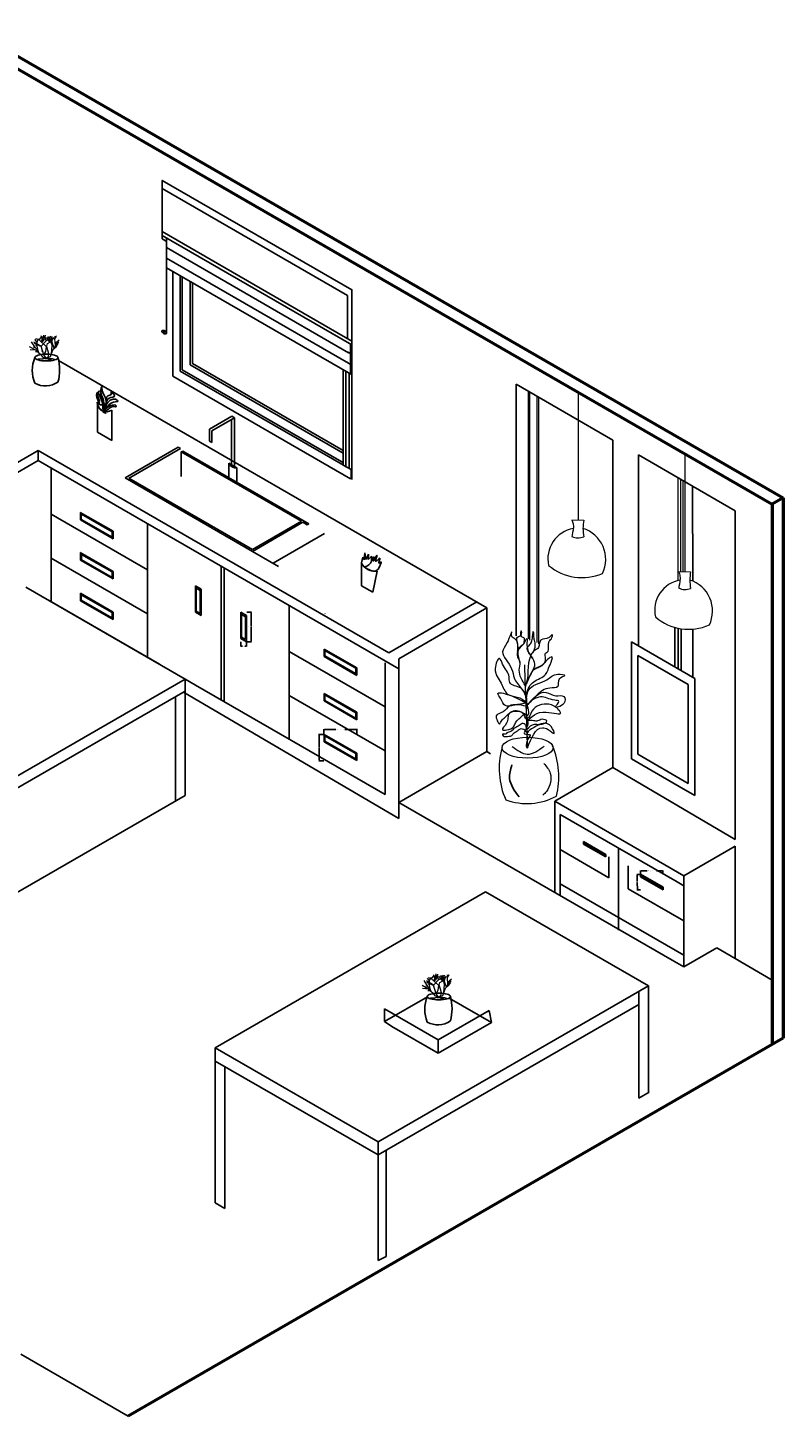
# Model space of a CAD drawing. Units: centimetres. Extents: x 5383 to 11288, y 5305 to 11515.
# Tile 4 of 5: x 5675 to 5972, y 5305 to 5851. Entities that reach past the tile are written whole.
import ezdxf

# ---------------------------------------------------------------- set-up
doc = ezdxf.new("R2010")
doc.units = ezdxf.units.CM
for name, color, linetype, lineweight in [('A-ANNO-DIMS', 2, 'Continuous', 18), ('A-FLOR-CASE', 3, 'Continuous', 25), ('A-FLOR-FIXT', 6, 'Continuous', 25), ('A-FURN', 8, 'Continuous', 25), ('A-FURN-PLNT', 82, 'Continuous', 13), ('A-GLAZ', 4, 'Continuous', 25), ('A-WALL', 7, 'Continuous', 50), ('E-LITE', 2, 'Continuous', 18)]:
    doc.layers.add(name, color=color, linetype=linetype, lineweight=lineweight)
doc.styles.get("Standard").update_dxf_attribs({"font": 'arial.ttf'})
doc.dimstyles.get("Standard").update_dxf_attribs({"dimtxt": 0.18, "dimasz": 0.18, "dimexe": 0.18, "dimexo": 0.0625, "dimgap": 0.09, "dimtad": 0, "dimtih": 1, "dimtoh": 1, "dimdec": 4, "dimzin": 0, "dimdsep": 46, "dimtxsty": 'Standard', "dimcen": 0.09, "dimadec": 0, "dimazin": 0, "dimtfac": 1, "dimtdec": 4, "dimtofl": 0, "dimtmove": 0, "dimatfit": 3, "dimfxl": 1, "dimtolj": 1, "dimtzin": 0, "dimarcsym": 0})

# ---------------------------------------------------------------- blocks, each defined once
blk = doc.blocks.new('*U2')
for p, q in [((-18.24, 11.04), (-21.755, 16.655)), ((-12.96, 12.48), (-19.68, 16.32)), ((-13.92, 12.48), (-19.2, 14.88)), ((-16.8, 16.32), (-18.72, 18.72)), ((-14.88, 18.24), (-17.76, 19.2)), ((-16.8, 12.48), (-17.76, 12.96)), ((-16.8, 16.32), (-15.36, 19.68)), ((-16.8, 12.48), (-16.8, 16.32)), ((-14.88, 18.24), (-12.96, 20.64)), ((-8.16, 12), (-14.88, 18.24)), ((-13.325, 16.724), (-11.433, 18.289)), ((-12.96, 12.48), (-8.16, 17.76)), ((-12.471, 19.775), (-12.898, 22.044)), ((-11.677, 19.071), (-12.471, 19.775)), ((-11.28, 19.619), (-12.104, 21.184)), ((-12.043, 15.628), (-11.921, 18.836)), ((-11.982, 16.802), (-10.579, 18.054)), ((-11.921, 18.836), (-10.64, 20.401)), ((-11.433, 18.289), (-10.457, 22.749)), ((-10.579, 18.054), (-9.846, 19.697)), ((-8.16, 17.76), (-10.56, 21.6)), ((-9.48, 19.775), (-8.992, 22.592)), ((-7.2, 19.68), (-8.64, 20.16)), ((-8.16, 17.76), (-5.28, 19.2)), ((-7.68, 12.48), (-7.2, 14.88)), ((-7.2, 19.68), (-6.24, 21.12)), ((-4.8, 16.32), (-7.2, 19.68)), ((-7.2, 14.88), (-3.84, 16.8)), ((-5.086, 17.741), (-5.513, 21.34)), ((-5.28, 19.2), (-3.84, 21.6)), ((-3.377, 15.315), (-5.086, 17.819)), ((-2.88, 12.96), (-4.32, 19.68)), ((-3.84, 16.8), (-0.96, 20.64)), ((-3.377, 18.602), (-2.888, 21.575)), ((-2.766, 16.802), (-3.377, 18.602)), ((-3.36, 5.28), (-2.88, 12.96)), ((-2.88, 15.84), (-2.4, 20.16)), ((-0.96, 10.56), (-2.88, 15.84)), ((-0.508, 21.888), (-0.081, 20.558)), ((-0.48, 10.8), (0.346, 13.203)), ((-0.203, 19.149), (0.102, 21.34)), ((0.346, 13.203), (-0.203, 19.149)), ((-0.142, 19.384), (0.59, 20.401)), ((-0.02, 20.01), (0.896, 21.105)), ((0.041, 20.714), (1.384, 22.044)), ((0.102, 21.34), (0.835, 21.888)), ((0.346, 13.203), (1.323, 16.254)), ((0.96, 12), (1.44, 15.36)), ((0.96, 12), (2.88, 14.88)), ((1.323, 16.254), (3.642, 18.289)), ((1.44, 15.36), (2.88, 17.28)), ((1.92, 13.44), (2.4, 15.36)), ((2.4, 15.36), (3.36, 16.32)), ((-17.76, 8.64), (-23.663, 11.961)), ((-17.76, 8.64), (-23.128, 9.222)), ((-18.24, 11.04), (-20.16, 11.52)), ((-15.84, 8.16), (-18.24, 11.04)), ((-16.32, 7.2), (-18.24, 7.2)), ((-14.88, 5.76), (-17.76, 8.64)), ((-15.84, 0.48), (-17.76, 0)), ((-15.84, 8.16), (-16.8, 12.48)), ((-14.88, 5.76), (-15.84, 8.16)), ((-13.44, 0.48), (-15.84, 0.48)), ((-12.96, 4.8), (-14.88, 5.76)), ((-12.96, 12.48), (-13.92, 12.48)), ((-9.6, 0.96), (-13.44, 0.48)), ((-10.56, 4.32), (-12.96, 12.48)), ((-11.52, 2.4), (-12.96, 4.8)), ((-9.6, 0.96), (-12.96, 0)), ((-8.64, 0.96), (-11.52, 2.4)), ((-10.56, 4.32), (-8.64, 7.68)), ((-8.64, 1.92), (-10.56, 4.32)), ((-9.6, 0.96), (-7.68, 0.96)), ((-8.64, 7.68), (-8.16, 12)), ((-8.64, 0.96), (-4.32, 2.88)), ((-8.64, 0.96), (-6.24, 2.88)), ((-8.64, 0.96), (-8.64, 1.92)), ((-8.64, 0.96), (-2.88, 0.96)), ((-6.72, 8.64), (-7.68, 12.48)), ((-7.68, 0.96), (-6.24, 0.48)), ((-5.76, 5.28), (-6.72, 8.64)), ((-6.24, 2.88), (-5.76, 5.28)), ((-6.24, 0.48), (-3.36, 0)), ((-4.32, 2.88), (-1.92, 9.6)), ((-2.88, 0.96), (0, 0)), ((-1.92, 9.6), (0.96, 12))]:
    blk.add_line(p, q)
blk = doc.blocks.new('HANDLE-DRAWER')
for p, q in [((12.85, 2.94), (0, 10.36)), ((0.01, 7.41), (0.01, 10.35)), ((0.01, 7.41), (12.85, 0)), ((0.4, 7.58), (0.4, 9.71)), ((12.49, 0.59), (0.4, 7.58)), ((0.5, 9.66), (12.49, 2.73)), ((12.49, 2.73), (12.49, 0.59)), ((12.85, 0), (12.85, 2.94))]:
    blk.add_line(p, q)
blk = doc.blocks.new('HANDLE-DRAWER-B')
for p, q in [((0, 6.1), (8.78, 1.03)), ((0, 6.1), (0, 5.07)), ((0.19, 5.78), (8.61, 0.92)), ((0.19, 5.78), (0.19, 5.23)), ((8.78, 0), (0, 5.07)), ((8.61, 0.37), (0.19, 5.23)), ((8.61, 0.92), (8.61, 0.37)), ((8.78, 1.03), (8.78, 0))]:
    blk.add_line(p, q)
blk = doc.blocks.new('HANDLE-DOOR-D')
for p, q in [((0, 11.69), (2.28, 10.37)), ((0, 1.32), (0, 11.69)), ((0.33, 10.73), (1.92, 9.81)), ((0.33, 1.75), (0.33, 10.73)), ((1.92, 9.81), (1.92, 0.83)), ((2.28, 10.37), (2.28, 0)), ((2.28, 0), (0, 1.32)), ((1.92, 0.83), (0.33, 1.75))]:
    blk.add_line(p, q)
blk = doc.blocks.new('*D16')
at = {"layer": 'A-ANNO-DIMS', "color": 0, "lineweight": -2, "transparency": 16777216}
for p, q in [((5791.14, 5573.38), (5791.14, 5575.42)), ((5791.32, 5575.24), (5795.82, 5575.25)), ((5803.82, 5575.25), (5799.32, 5575.25)), ((5804, 5573.39), (5804, 5575.43))]:
    blk.add_line(p, q, dxfattribs=at)
at = {"layer": 'A-ANNO-DIMS', "color": 0, "transparency": 16777216}
for points in [[(5791.32, 5575.27), (5791.32, 5575.21), (5791.14, 5575.24)], [(5803.82, 5575.28), (5803.82, 5575.22), (5804, 5575.25)]]:
    blk.add_solid(points, dxfattribs=at)
at = {"layer": 'Defpoints', "color": 0, "transparency": 16777216}
for p in [(5791.14, 5575.24), (5791.14, 5573.32), (5804, 5573.33)]:
    blk.add_point(p, dxfattribs=at)
at = {"layer": 'A-ANNO-DIMS', "color": 0, "transparency": 16777216, "insert": (5797.57, 5575.25), "char_height": 0.18, "attachment_point": 5}
blk.add_mtext('\\A1;HANDLE (DRAWER) 13 TYP.', dxfattribs=at)
blk = doc.blocks.new('*D17')
at = {"layer": 'A-ANNO-DIMS', "color": 0, "lineweight": -2, "transparency": 16777216}
for p, q in [((5791.08, 5573.32), (5789.04, 5573.31)), ((5789.22, 5573.13), (5789.22, 5568.32)), ((5789.22, 5563.13), (5789.22, 5567.95)), ((5791.09, 5562.96), (5789.05, 5562.95))]:
    blk.add_line(p, q, dxfattribs=at)
at = {"layer": 'A-ANNO-DIMS', "color": 0, "transparency": 16777216}
for points in [[(5789.25, 5573.13), (5789.19, 5573.13), (5789.22, 5573.31)], [(5789.25, 5563.13), (5789.19, 5563.13), (5789.23, 5562.95)]]:
    blk.add_solid(points, dxfattribs=at)
at = {"layer": 'Defpoints', "color": 0, "transparency": 16777216}
for p in [(5791.14, 5573.32), (5789.23, 5562.95), (5791.15, 5562.96)]:
    blk.add_point(p, dxfattribs=at)
at = {"layer": 'A-ANNO-DIMS', "color": 0, "transparency": 16777216, "insert": (5789.22, 5568.13), "char_height": 0.18, "attachment_point": 5}
blk.add_mtext('\\A1;10 TYP.', dxfattribs=at)
blk = doc.blocks.new('*D24')
at = {"layer": 'A-ANNO-DIMS', "color": 0, "lineweight": -2, "transparency": 16777216}
for p, q in [((5915.66, 5518.31), (5915.66, 5519.74)), ((5915.84, 5519.56), (5918.25, 5519.57)), ((5924.26, 5519.61), (5921.84, 5519.59)), ((5924.44, 5518.35), (5924.44, 5519.79))]:
    blk.add_line(p, q, dxfattribs=at)
at = {"layer": 'A-ANNO-DIMS', "color": 0, "transparency": 16777216}
for points in [[(5915.84, 5519.59), (5915.84, 5519.53), (5915.66, 5519.56)], [(5924.26, 5519.64), (5924.26, 5519.58), (5924.44, 5519.61)]]:
    blk.add_solid(points, dxfattribs=at)
at = {"layer": 'Defpoints', "color": 0, "transparency": 16777216}
for p in [(5915.66, 5519.56), (5915.66, 5518.24), (5924.44, 5518.29)]:
    blk.add_point(p, dxfattribs=at)
at = {"layer": 'A-ANNO-DIMS', "color": 0, "transparency": 16777216, "insert": (5920.05, 5519.58), "char_height": 0.18, "attachment_point": 5}
blk.add_mtext('\\A1;HANDLE (DRAWER B) 9 TYP.', dxfattribs=at)
blk = doc.blocks.new('*D25')
at = {"layer": 'A-ANNO-DIMS', "color": 0, "lineweight": -2, "transparency": 16777216}
for p, q in [((5915.6, 5518.24), (5914.17, 5518.23)), ((5914.35, 5518.06), (5914.36, 5515.37)), ((5914.38, 5512.32), (5914.36, 5515.01)), ((5915.63, 5512.15), (5914.2, 5512.14))]:
    blk.add_line(p, q, dxfattribs=at)
at = {"layer": 'A-ANNO-DIMS', "color": 0, "transparency": 16777216}
for points in [[(5914.38, 5518.06), (5914.32, 5518.06), (5914.35, 5518.24)], [(5914.41, 5512.32), (5914.35, 5512.32), (5914.38, 5512.14)]]:
    blk.add_solid(points, dxfattribs=at)
at = {"layer": 'Defpoints', "color": 0, "transparency": 16777216}
for p in [(5915.66, 5518.24), (5914.38, 5512.14), (5915.7, 5512.15)]:
    blk.add_point(p, dxfattribs=at)
at = {"layer": 'A-ANNO-DIMS', "color": 0, "transparency": 16777216, "insert": (5914.36, 5515.19), "char_height": 0.18, "attachment_point": 5}
blk.add_mtext('\\A1;6 TYP.', dxfattribs=at)
blk = doc.blocks.new('*D26')
at = {"layer": 'A-ANNO-DIMS', "color": 0, "lineweight": -2, "transparency": 16777216}
for p, q in [((5760.76, 5621.46), (5762.63, 5621.46)), ((5762.45, 5621.28), (5762.45, 5615.79)), ((5762.45, 5609.95), (5762.45, 5615.43)), ((5760.76, 5609.77), (5762.63, 5609.77))]:
    blk.add_line(p, q, dxfattribs=at)
at = {"layer": 'A-ANNO-DIMS', "color": 0, "transparency": 16777216}
for points in [[(5762.42, 5621.28), (5762.48, 5621.28), (5762.45, 5621.46)], [(5762.42, 5609.95), (5762.48, 5609.95), (5762.45, 5609.77)]]:
    blk.add_solid(points, dxfattribs=at)
at = {"layer": 'Defpoints', "color": 0, "transparency": 16777216}
for p in [(5760.7, 5621.46), (5762.45, 5621.46), (5760.7, 5609.77)]:
    blk.add_point(p, dxfattribs=at)
at = {"layer": 'A-ANNO-DIMS', "color": 0, "transparency": 16777216, "insert": (5762.45, 5615.61), "char_height": 0.18, "attachment_point": 5}
blk.add_mtext('\\A1;HANDLE D 12 TYP.', dxfattribs=at)
blk = doc.blocks.new('*D27')
at = {"layer": 'A-ANNO-DIMS', "color": 0, "lineweight": -2, "transparency": 16777216}
for p, q in [((5758.41, 5609.71), (5758.41, 5607.84)), ((5758.59, 5608.02), (5759.09, 5608.02)), ((5760.52, 5608.02), (5760.01, 5608.02)), ((5760.7, 5609.71), (5760.7, 5607.84))]:
    blk.add_line(p, q, dxfattribs=at)
at = {"layer": 'A-ANNO-DIMS', "color": 0, "transparency": 16777216}
for points in [[(5758.59, 5608.05), (5758.59, 5607.99), (5758.41, 5608.02)], [(5760.52, 5608.05), (5760.52, 5607.99), (5760.7, 5608.02)]]:
    blk.add_solid(points, dxfattribs=at)
at = {"layer": 'Defpoints', "color": 0, "transparency": 16777216}
for p in [(5758.41, 5609.77), (5760.7, 5609.77), (5760.7, 5608.02)]:
    blk.add_point(p, dxfattribs=at)
at = {"layer": 'A-ANNO-DIMS', "color": 0, "transparency": 16777216, "insert": (5759.55, 5608.02), "char_height": 0.18, "attachment_point": 5}
blk.add_mtext('\\A1;2 TYP.', dxfattribs=at)

msp = doc.modelspace()

# ---------------------------------------------------------------- linework, layer by layer
at = {"layer": 'A-FLOR-CASE'}
for p, q in [((5678.77, 5725.01), (5678.79, 5725.03)), ((5680, 5724.33), (5680.45, 5724.06)), ((5686.8, 5720.4), (5855.22, 5623.16)), ((5866.77, 5622.62), (5866.77, 5711.16)), ((5866.77, 5711.16), (5904.77, 5689.1)), ((5702.01, 5704.03), (5702.01, 5692.28)), ((5707.72, 5688.98), (5707.72, 5700.91)), ((5702.01, 5692.28), (5707.72, 5688.98)), ((5904.77, 5686.2), (5904.77, 5689.1)), ((5575.44, 5625.3), (5678.79, 5684.97)), ((5678.79, 5681.05), (5678.79, 5684.97)), ((5678.79, 5684.97), (5816.59, 5605.41)), ((5904.77, 5686.2), (5904.77, 5560.27)), ((5914.77, 5683.3), (5914.77, 5608.1)), ((5914.77, 5683.3), (5952.78, 5661.23)), ((5575.44, 5621.38), (5678.79, 5681.05)), ((5678.79, 5681.05), (5820.61, 5599.16)), ((5683.84, 5678.13), (5683.84, 5625.49)), ((5936.1, 5670.91), (5936.17, 5633.61)), ((5683.84, 5659.91), (5721.78, 5638)), ((5708.17, 5653.2), (5695.32, 5660.62)), ((5695.33, 5657.67), (5695.33, 5660.61)), ((5695.71, 5657.83), (5695.71, 5659.97)), ((5695.71, 5659.97), (5695.81, 5659.91)), ((5695.81, 5659.91), (5707.81, 5652.99)), ((5952.78, 5661.23), (5952.78, 5531.97)), ((5695.33, 5657.67), (5708.17, 5650.26)), ((5707.81, 5650.85), (5695.71, 5657.83)), ((5721.78, 5656.22), (5721.78, 5603.58)), ((5707.81, 5652.99), (5707.81, 5650.85)), ((5708.17, 5650.26), (5708.17, 5653.2)), ((5806.95, 5641.99), (5807.23, 5644.68)), ((5807.23, 5644.68), (5807.6, 5642.18)), ((5807.6, 5642.18), (5808.68, 5644.25)), ((5808.68, 5644.25), (5808.55, 5642.08)), ((5808.55, 5642.08), (5809.86, 5643.46)), ((5809.86, 5643.46), (5809.8, 5641.5)), ((5683.84, 5642.7), (5721.78, 5620.79)), ((5750.64, 5639.56), (5750.64, 5586.92)), ((5751.89, 5638.84), (5751.89, 5586.2)), ((5805.85, 5640.82), (5806.37, 5643)), ((5805.85, 5640.82), (5805.85, 5631.8)), ((5806.37, 5643), (5806.95, 5641.99)), ((5812.07, 5637.58), (5810.32, 5629.21)), ((5673.95, 5631.2), (5736.51, 5595.08)), ((5805.85, 5631.8), (5810.32, 5629.21)), ((5683.06, 5625.94), (5726.46, 5600.88)), ((5777.44, 5624.09), (5777.44, 5571.45)), ((5816.59, 5605.41), (5851.28, 5625.44)), ((5855.22, 5623.16), (5820.61, 5603.09)), ((5855.22, 5623.16), (5855.22, 5566.51)), ((5866.77, 5622.62), (5866.77, 5612.08)), ((5791.51, 5620.82), (5791.61, 5620.76)), ((5929.1, 5615.44), (5929.1, 5599.83)), ((5930.48, 5615.1), (5930.48, 5599.03)), ((5931.63, 5614.9), (5931.63, 5598.37)), ((5936.17, 5614.74), (5936.17, 5595.75)), ((5777.44, 5605.87), (5815.15, 5584.1)), ((5936.96, 5595.29), (5912.01, 5609.7)), ((5912.01, 5609.7), (5912.01, 5563.63)), ((5815.15, 5601.43), (5815.15, 5549.68)), ((5820.61, 5603.09), (5820.61, 5599.16)), ((5914.53, 5604.41), (5934.41, 5592.93)), ((5914.53, 5565.49), (5914.53, 5604.41)), ((5736.51, 5595.08), (5620.89, 5528.33)), ((5740.66, 5592.69), (5736.22, 5595.24)), ((5736.51, 5595.08), (5738.15, 5594.13)), ((5736.51, 5595.08), (5736.51, 5549.21)), ((5820.61, 5599.16), (5820.61, 5546.52)), ((5936.96, 5549.23), (5936.96, 5595.29)), ((5620.89, 5523.54), (5736.51, 5590.29)), ((5738.15, 5588.61), (5735.87, 5589.92)), ((5740.66, 5592.69), (5815.15, 5549.68)), ((5934.41, 5592.93), (5934.41, 5554.01)), ((5732.81, 5588.15), (5732.81, 5547.08)), ((5820.61, 5540.21), (5738.15, 5588.61)), ((5777.44, 5588.66), (5815.15, 5566.89)), ((5820.61, 5546.52), (5855.22, 5566.51)), ((5855.22, 5566.51), (5856.64, 5565.68)), ((5912.01, 5563.63), (5930.86, 5552.75)), ((5934.41, 5554.01), (5914.53, 5565.49)), ((5904.77, 5560.27), (5881.87, 5547.04)), ((5904.77, 5560.27), (5952.78, 5531.97)), ((5930.86, 5552.75), (5936.96, 5549.23)), ((5640.52, 5493.8), (5736.51, 5549.21)), ((5820.61, 5546.52), (5820.61, 5540.21)), ((5820.61, 5546.52), (5928.12, 5484.45)), ((5881.87, 5547.04), (5932.67, 5517.71)), ((5881.87, 5547.04), (5881.87, 5511.16)), ((5884.02, 5541.81), (5884.02, 5509.91)), ((5884.02, 5541.81), (5929.98, 5515.28)), ((5952.78, 5529.32), (5932.67, 5517.71)), ((5952.78, 5529.32), (5952.78, 5508.19)), ((5884.02, 5528), (5903.21, 5516.93)), ((5903.21, 5516.93), (5903.21, 5525.17)), ((5907, 5528.55), (5907, 5496.32)), ((5910.7, 5512.6), (5910.7, 5521.56)), ((5884.02, 5514.52), (5932.67, 5486.43)), ((5910.7, 5512.6), (5932.67, 5499.92)), ((5929.98, 5515.28), (5932.67, 5513.73)), ((5932.67, 5517.71), (5932.67, 5481.83)), ((5952.78, 5508.19), (5952.78, 5485.1)), ((5932.67, 5481.83), (5945.56, 5489.27)), ((5952.78, 5485.1), (5945.56, 5489.27)), ((5952.78, 5485.1), (5967.4, 5476.66)), ((5932.67, 5481.83), (5928.12, 5484.45)), ((5831.8, 5470.03), (5814.91, 5460.28)), ((5834.21, 5471.43), (5834.06, 5471.34)), ((5837.25, 5471.37), (5837.02, 5471.5)), ((5856.99, 5459.97), (5840.35, 5469.58)), ((5812.41, 5407.82), (5914.96, 5467.02)), ((5814.91, 5460.28), (5814.91, 5465.32)), ((5814.91, 5465.32), (5836.04, 5453.07)), ((5836.04, 5453.07), (5856.12, 5464.66)), ((5856.12, 5464.66), (5856.99, 5459.97)), ((5814.91, 5460.28), (5817.86, 5458.37)), ((5817.86, 5458.37), (5836.04, 5447.87)), ((5836.04, 5447.87), (5856.99, 5459.97)), ((5836.04, 5447.87), (5836.04, 5453.07)), ((5748.33, 5444.76), (5812.41, 5407.82)), ((5671.93, 5329.42), (5714.19, 5305.03))]:
    msp.add_line(p, q, dxfattribs=at)
for centre, radius, start, end in [((5689.43, 5716.53), 13, 157.2197, 202.7803), ((5668.39, 5716.74), 18.77, 345.1121, 14.8879), ((5681.64, 5719.12), 8.7, 241.172, 304.1782), ((5705.67, 5703.94), 3.67, 178.6934, 304.0622), ((5811.23, 5643.57), 6.05, 207.0835, 277.9309), ((5806.55, 5642.61), 3.43, 278.1771, 341.0356), ((5843.76, 5465.15), 13, 157.2197, 202.7803), ((5822.71, 5465.36), 18.77, 345.1121, 14.8879), ((5835.96, 5467.74), 8.7, 241.172, 304.1782)]:
    msp.add_arc(centre, radius, start, end, dxfattribs=at)
for centre in [(5681.99, 5721.56), (5836.31, 5470.18)]:
    msp.add_ellipse(centre, major_axis=(-4.54, 0), ratio=0.292852, dxfattribs=at)
for points, knots in [([(5704.58, 5703.7), (5704.47, 5704.47), (5704.24, 5706.01), (5703.13, 5707.37), (5703.66, 5710.77), (5703.89, 5709.13), (5703.95, 5707.59), (5706.07, 5705.03), (5705.17, 5702.17), (5704.73, 5700.61), (5704.67, 5700.42)], [0, 0, 0, 0, 2.2262, 4.397419, 6.485307, 7.045711, 8.305236, 11.539925, 15.801023, 16.419307, 16.419307, 16.419307, 16.419307]), ([(5704.16, 5701.93), (5704.26, 5702.28), (5704.49, 5703.13), (5702.54, 5702.63), (5703.17, 5705.32), (5701.51, 5706.54), (5703.16, 5708.91), (5701.27, 5707.12), (5702.01, 5705.71), (5702.46, 5704.11), (5702.07, 5702.6), (5703.03, 5701.33), (5703.87, 5700.54), (5704.98, 5700.44), (5705.01, 5699.38), (5705.41, 5699.68), (5705.51, 5699.75)], [0, 0, 0, 0, 0.857723, 2.078573, 3.423978, 6.729409, 7.621637, 8.998179, 10.743822, 12.288797, 13.957052, 15.003163, 16.876499, 17.219162, 18.157501, 18.478065, 18.478065, 18.478065, 18.478065]), ([(5704.41, 5700.5), (5704.29, 5700.82), (5704.06, 5701.44), (5704.35, 5702.97), (5703.72, 5704.44), (5702.34, 5708.43), (5704.06, 5705.2), (5704.79, 5703.35), (5704.98, 5701.36), (5704.73, 5700.39), (5704.72, 5700.39)], [0, 0, 0, 0, 1.020009, 1.960922, 4.409418, 6.98547, 8.907748, 11.263854, 14.254879, 14.267247, 14.267247, 14.267247, 14.267247]), ([(5704.84, 5701.01), (5705.58, 5701.97), (5706.88, 5703.65), (5708.8, 5704.15), (5710.35, 5704.3), (5709.3, 5705.33), (5708.15, 5705.21), (5706.02, 5704.42), (5705.04, 5702.34), (5704.85, 5700.55), (5704.48, 5700.05), (5704.31, 5699.82)], [0, 0, 0, 0, 3.437706, 6.040469, 6.373078, 7.295495, 8.501484, 10.177458, 13.696544, 14.666719, 15.508627, 15.508627, 15.508627, 15.508627]), ([(5705.52, 5703.1), (5705.62, 5704.12), (5705.81, 5705.99), (5710.09, 5705.91), (5707, 5708.59), (5707.7, 5706.78), (5705.43, 5706.72), (5705.54, 5704.37), (5705.33, 5703.05), (5705.23, 5702.44)], [0, 0, 0, 0, 2.740578, 5.054316, 6.922776, 7.52988, 9.028676, 11.251258, 13.187584, 13.187584, 13.187584, 13.187584]), ([(5704.72, 5700.39), (5705.3, 5700.66), (5706.56, 5701.26), (5707.64, 5702.54), (5709.72, 5702.05), (5709.15, 5703.03), (5708.24, 5702.78), (5706.43, 5702.8), (5705.42, 5701.42), (5704.67, 5700.42)], [0, 0, 0, 0, 1.871313, 4.116624, 5.181401, 5.718262, 6.471186, 7.710974, 11.104157, 11.104157, 11.104157, 11.104157]), ([(5807.04, 5639.21), (5808.56, 5638.24), (5811.26, 5636.52), (5812.95, 5638.9), (5813.89, 5641.64), (5812.04, 5639.83), (5814.04, 5644.21), (5810.44, 5639.59), (5813.09, 5646.2), (5810.43, 5640.74), (5810.42, 5642.19), (5811.61, 5644.07), (5809.32, 5642.02), (5809.89, 5642.03), (5809.93, 5642.03)], [0, 0, 0, 0, 4.519716, 8.015938, 8.952883, 9.857618, 11.754396, 13.722919, 16.068694, 18.673826, 18.815379, 20.24018, 21.699493, 21.816492, 21.816492, 21.816492, 21.816492]), ([(5865.01, 5561.3), (5864.49, 5559.48), (5863.18, 5554.92), (5866.12, 5551.03), (5867.9, 5548.69)], [0, 0, 0, 0, 5.435763, 13.608405, 13.608405, 13.608405, 13.608405])]:
    msp.add_open_spline(points, degree=3, knots=knots, dxfattribs=at)
at = {"layer": 'A-FLOR-FIXT'}
for p, q in [((5754.93, 5698.48), (5746.11, 5693.39)), ((5755.98, 5697.87), (5754.93, 5698.48)), ((5746.11, 5693.39), (5746.11, 5688.64)), ((5755.98, 5697.87), (5747.07, 5692.73)), ((5747.07, 5692.73), (5747.07, 5688.57)), ((5754.76, 5678.69), (5754.76, 5697.16)), ((5755.98, 5678.19), (5755.98, 5697.87)), ((5746.11, 5688.64), (5746.97, 5688.15)), ((5746.97, 5688.15), (5747.07, 5688.09)), ((5747.07, 5688.57), (5747.07, 5688.09)), ((5733.82, 5686.28), (5712.92, 5674.22)), ((5734.68, 5685.79), (5715.24, 5674.57)), ((5733.82, 5686.28), (5734.68, 5685.79)), ((5735.02, 5684.43), (5735.61, 5684.76)), ((5735.02, 5684.43), (5782.29, 5657.14)), ((5735.02, 5684.43), (5735.02, 5674.74)), ((5735.61, 5684.76), (5785.16, 5656.15)), ((5753.77, 5674.28), (5753.77, 5679.99)), ((5753.77, 5679.99), (5756.87, 5678.2)), ((5756.87, 5678.2), (5756.87, 5672.48)), ((5712.92, 5674.22), (5762.98, 5645.31)), ((5714.45, 5674.11), (5715.24, 5674.57)), ((5714.45, 5674.11), (5763.07, 5646.04)), ((5762.98, 5645.31), (5782.87, 5656.8)), ((5763.07, 5646.04), (5782.29, 5657.14)), ((5782.87, 5656.8), (5784.58, 5655.82)), ((5784.58, 5655.82), (5785.16, 5656.15)), ((5771.11, 5640.62), (5791.39, 5652.33)), ((5762.98, 5645.31), (5773.28, 5639.37))]:
    msp.add_line(p, q, dxfattribs=at)
msp.add_arc((5756.4, 5680.96), 2.8, 200.1749, 279.8251, dxfattribs=at)
at = {"layer": 'A-FURN'}
for p, q in [((5854.63, 5511.33), (5748.33, 5449.96)), ((5918.72, 5474.33), (5854.63, 5511.33)), ((5812.41, 5412.96), (5918.72, 5474.33)), ((5918.72, 5474.33), (5918.72, 5432.63)), ((5914.96, 5472.16), (5914.96, 5430.14)), ((5748.33, 5449.96), (5812.41, 5412.96)), ((5748.33, 5449.96), (5748.33, 5389.05)), ((5752.15, 5442.55), (5752.15, 5386.76)), ((5914.96, 5430.14), (5919, 5432.47)), ((5918.72, 5432.63), (5919, 5432.47)), ((5812.41, 5412.96), (5812.41, 5366.25)), ((5815.56, 5409.63), (5815.56, 5367.86)), ((5752.15, 5386.76), (5752.15, 5395.88)), ((5752.15, 5386.76), (5748.33, 5389.05)), ((5815.56, 5367.86), (5812.41, 5366.25))]:
    msp.add_line(p, q, dxfattribs=at)
at = {"layer": 'A-FURN-PLNT'}
for centre, radius, start, end in [((5890.23, 5559.8), 30.2, 164.3402, 203.7975), ((5850.89, 5556.55), 32.58, 346.6593, 22.1857), ((5871.06, 5570), 23.93, 249.3073, 298.8064)]:
    msp.add_arc(centre, radius, start, end, dxfattribs=at)
msp.add_ellipse((5871.19, 5568.07), major_axis=(-10.04, 0), ratio=0.411404, dxfattribs=at)
for points, knots in [([(5868.27, 5601.23), (5867.89, 5602.75), (5867.11, 5605.83), (5867.67, 5610.68), (5864.53, 5611.57), (5865.42, 5615.48), (5863.28, 5608.65), (5859.83, 5605.19), (5865.23, 5600.42), (5865.67, 5594.9), (5868.48, 5591.75), (5871.01, 5588.26), (5870.78, 5585.74), (5870.65, 5584.35)], [0, 0, 0, 0, 4.887819, 9.955609, 11.466226, 13.131437, 17.60703, 21.579314, 29.227498, 32.917957, 38.122483, 41.415032, 45.430736, 45.430736, 45.430736, 45.430736]), ([(5867.43, 5606.05), (5867.46, 5607.03), (5867.5, 5608.74), (5866.49, 5611.92), (5869.15, 5611.91), (5868.69, 5615.37), (5868.06, 5611.61), (5870.03, 5611.46), (5869.76, 5609.95), (5869.74, 5608.49), (5867.95, 5608.13), (5866.58, 5605.5), (5867.55, 5605.6), (5867.59, 5605.61)], [0, 0, 0, 0, 3.174057, 5.569375, 7.256431, 8.890822, 11.014836, 12.391144, 13.272783, 15.059197, 16.05349, 18.742928, 18.876438, 18.876438, 18.876438, 18.876438]), ([(5870.38, 5592.45), (5871.18, 5594.29), (5872.37, 5597.04), (5874.56, 5601.02), (5872.25, 5604.6), (5870.62, 5606.92), (5871.24, 5612.3), (5869.64, 5608.39), (5867.76, 5607.28), (5866.75, 5604.22), (5868.78, 5601.7), (5867.21, 5597.3), (5869.1, 5594.41), (5870.38, 5592.45)], [0, 0, 0, 0, 6.159679, 9.221838, 12.563186, 17.326771, 19.858712, 22.189415, 24.928377, 27.481367, 30.452133, 33.593987, 40.15181, 40.15181, 40.15181, 40.15181]), ([(5873.54, 5598.7), (5874.12, 5599.05), (5875.22, 5599.71), (5876.88, 5600.28), (5878.21, 5601.67), (5878.38, 5603.39), (5877.83, 5605.27), (5879.48, 5605.77), (5879.48, 5607.77), (5879.26, 5609.97), (5880.84, 5610.89), (5881.14, 5613.17), (5879.18, 5610.32), (5876.72, 5611.36), (5875.74, 5609.09), (5875.83, 5607.17), (5873.57, 5606.33), (5870.54, 5601.57), (5871.91, 5595.92), (5870.38, 5592.45)], [0, 0, 0, 0, 2.047288, 3.821296, 5.229817, 7.484976, 8.975351, 9.972137, 11.695465, 14.210894, 15.978215, 17.094508, 18.691023, 21.967989, 23.491175, 25.160962, 27.300555, 29.670695, 41.707533, 41.707533, 41.707533, 41.707533]), ([(5872.42, 5604.31), (5872.12, 5604.8), (5871.59, 5605.69), (5870.68, 5607.43), (5872.27, 5608.51), (5873.05, 5610.43), (5873.17, 5611.8), (5873.47, 5614.47), (5873.51, 5611.76), (5873.76, 5610.36), (5874.35, 5607.86), (5873.56, 5605.89), (5872.04, 5604.28), (5872.8, 5603.51), (5873.19, 5603.11)], [0, 0, 0, 0, 1.770718, 3.264142, 4.976902, 6.600288, 9.225814, 10.325743, 11.832972, 13.768893, 15.968751, 18.850787, 20.173552, 21.598942, 21.598942, 21.598942, 21.598942]), ([(5870.52, 5588.37), (5870.08, 5589.56), (5869.02, 5592.41), (5863.65, 5592.38), (5864.3, 5597.42), (5861.75, 5599.4), (5859.96, 5604.93), (5857.35, 5597.45), (5860.97, 5594.3), (5863.02, 5586.92), (5871.13, 5589.56), (5871.95, 5579.85), (5870.59, 5580.91), (5870.5, 5580.98)], [0, 0, 0, 0, 3.602126, 8.634898, 10.866263, 16.477372, 19.011704, 23.341676, 29.567945, 34.443269, 42.833484, 47.400461, 47.734568, 47.734568, 47.734568, 47.734568]), ([(5870.52, 5588.37), (5871.08, 5590.34), (5872.17, 5594.21), (5878.52, 5595.84), (5879.43, 5599.59), (5881.76, 5604.7), (5878.3, 5602.47), (5877.23, 5600.04), (5873.29, 5599.35), (5871.83, 5595.79), (5869.66, 5591.81), (5870.86, 5587.23), (5870.7, 5583.39), (5870.66, 5579.88), (5872.13, 5577.06), (5868.65, 5572.97), (5873.5, 5573.55), (5870.36, 5571.33), (5870.58, 5567.28), (5871.31, 5568.2), (5871.37, 5568.28)], [0, 0, 0, 0, 5.811918, 11.386033, 16.172585, 19.324364, 21.379612, 24.581427, 27.8312, 31.736395, 35.307362, 41.24559, 44.939878, 46.977115, 51.620327, 54.398227, 56.668812, 59.025332, 62.038122, 62.318112, 62.318112, 62.318112, 62.318112]), ([(5870.65, 5584.35), (5872.03, 5585.84), (5874.72, 5588.75), (5878.49, 5592.01), (5884, 5591.27), (5882.53, 5595.41), (5887.31, 5596.58), (5881.53, 5597.56), (5878.8, 5593.76), (5870.67, 5592.75), (5870.66, 5587.15), (5870.65, 5584.35)], [0, 0, 0, 0, 6.083388, 11.846279, 15.054234, 18.06111, 20.624872, 23.314815, 28.221536, 35.581499, 42.924421, 42.924421, 42.924421, 42.924421]), ([(5870.61, 5585.6), (5868.87, 5586.66), (5866.1, 5588.35), (5858.26, 5590.47), (5861.08, 5587.02), (5861.95, 5583.9), (5865.38, 5584.74), (5867.99, 5585.12), (5869.64, 5585.42), (5870.61, 5585.6)], [0, 0, 0, 0, 7.459531, 11.853126, 14.165048, 17.403796, 20.663431, 22.713288, 25.647633, 25.647633, 25.647633, 25.647633]), ([(5870.65, 5584.35), (5871.47, 5585.36), (5872.93, 5587.17), (5877.36, 5588.67), (5879.89, 5586.81), (5884.64, 5586.53), (5880.2, 5583), (5886.4, 5584.77), (5885.89, 5589.16), (5881.79, 5587.92), (5876.84, 5591.71), (5873.22, 5587.41), (5870.65, 5584.35)], [0, 0, 0, 0, 3.874847, 6.924527, 12.695448, 14.373575, 16.910195, 20.490617, 23.221432, 26.452299, 30.366404, 39.966461, 39.966461, 39.966461, 39.966461]), ([(5870.65, 5584.35), (5869.47, 5584.63), (5867.35, 5585.13), (5863.63, 5584.85), (5862.14, 5581.84), (5858.23, 5581.17), (5859.17, 5578.97), (5860.17, 5576.67), (5860.79, 5578.79), (5862.32, 5579.84), (5864.13, 5582.15), (5867.21, 5582.74), (5869.19, 5581.89), (5870.8, 5581.14), (5870.61, 5580.06), (5870.51, 5579.53)], [0, 0, 0, 0, 3.692788, 6.645493, 10.089059, 13.209731, 15.170324, 16.789696, 17.945671, 19.773672, 22.795413, 26.342308, 28.012166, 29.487789, 30.943219, 30.943219, 30.943219, 30.943219]), ([(5870.86, 5578.06), (5872.7, 5580.23), (5875.74, 5583.81), (5885.37, 5580.4), (5882.76, 5584.04), (5878.96, 5585.99), (5872.84, 5584.4), (5871.93, 5579.52), (5870.61, 5579.53), (5870.51, 5579.53)], [0, 0, 0, 0, 8.683556, 14.311899, 15.470514, 20.075569, 27.209432, 30.783322, 31.080603, 31.080603, 31.080603, 31.080603]), ([(5870.51, 5579.53), (5870.09, 5580.52), (5868.99, 5583.08), (5862.72, 5582.4), (5864.06, 5578.07), (5860.16, 5574.78), (5863.68, 5575.12), (5865.7, 5575.73), (5866.42, 5578.1), (5867.81, 5579.43), (5871.25, 5582.93), (5870.46, 5578.11), (5871.36, 5578.54), (5871.43, 5578.58)], [0, 0, 0, 0, 3.07945, 7.891689, 11.911074, 14.934309, 16.619315, 19.584714, 21.342078, 23.254328, 26.469617, 29.063271, 29.284988, 29.284988, 29.284988, 29.284988]), ([(5870.95, 5575.33), (5871.9, 5576.27), (5873.41, 5577.78), (5876.05, 5576.82), (5880.14, 5578.45), (5876.74, 5579.63), (5875.3, 5578.38), (5873.44, 5578.72), (5870.87, 5579.06), (5870.9, 5577.16), (5870.92, 5576.14)], [0, 0, 0, 0, 3.542456, 5.63773, 8.76948, 10.722859, 12.609315, 14.172956, 16.336216, 18.819607, 18.819607, 18.819607, 18.819607]), ([(5871.19, 5568.07), (5872.69, 5571.94), (5874.56, 5576.75), (5879.38, 5575.57), (5882.46, 5572.31), (5880.6, 5577.23), (5877.26, 5578.11), (5874.15, 5576.15), (5870.77, 5574.64), (5870.97, 5572.67), (5871.02, 5572.2)], [0, 0, 0, 0, 9.793457, 12.199879, 15.003845, 17.920537, 21.377633, 24.650104, 28.978037, 30.323705, 30.323705, 30.323705, 30.323705]), ([(5870.78, 5575.85), (5870.67, 5576.37), (5870.52, 5577.17), (5869.14, 5577.88), (5867.9, 5576.49), (5865.97, 5576.06), (5864.88, 5574.19), (5863.15, 5574.24), (5862.51, 5573.04), (5861.16, 5573.78), (5861.56, 5572.41), (5863.1, 5572.54), (5864.83, 5572.46), (5865.93, 5574.02), (5867.15, 5574.62), (5867.98, 5575.28), (5868.79, 5575.7), (5869.35, 5575.41), (5869.98, 5575.36), (5870.17, 5574.52), (5871.16, 5574.14), (5870.94, 5573.38), (5870.99, 5572.46), (5871.08, 5571.58), (5871.1, 5570.82), (5871.1, 5570.68)], [0, 0, 0, 0, 1.526269, 2.318636, 4.069995, 6.140734, 8.204822, 9.786821, 10.661348, 11.663203, 12.342047, 13.402479, 15.812764, 17.206773, 18.752004, 19.821823, 20.437322, 21.311605, 21.575079, 22.236328, 23.466045, 24.029516, 24.362016, 26.255175, 26.654698, 26.654698, 26.654698, 26.654698]), ([(5865.13, 5568.58), (5867.11, 5567.1), (5871.26, 5563.98), (5875.5, 5567.07), (5877.71, 5568.69)], [0, 0, 0, 0, 6.702447, 14.027725, 14.027725, 14.027725, 14.027725]), ([(5877.53, 5561.9), (5878.59, 5560.69), (5881.31, 5557.59), (5879.94, 5552.02), (5877.72, 5549.86), (5877.23, 5549.39)], [0, 0, 0, 0, 4.654944, 11.957601, 13.995504, 13.995504, 13.995504, 13.995504])]:
    msp.add_open_spline(points, degree=3, knots=knots, dxfattribs=at)
msp.add_open_spline([(5871.19, 5568.07), (5870.83, 5578.93), (5870.47, 5589.78), (5870.11, 5600.63)], degree=3, dxfattribs=at)
at = {"layer": 'A-GLAZ'}
for p, q in [((5727.51, 5788.03), (5800.37, 5746.01)), ((5728.78, 5767.55), (5729.21, 5767.3)), ((5729.21, 5768.63), (5729.21, 5756.93)), ((5729.21, 5760.65), (5800.8, 5719.32)), ((5735.37, 5753.38), (5735.37, 5718.09)), ((5800.37, 5745.36), (5800.37, 5746.01)), ((5800.37, 5745.36), (5800.37, 5729.07)), ((5801.8, 5726.72), (5801.8, 5715.02)), ((5735.37, 5718.09), (5735.37, 5716.77)), ((5801.01, 5715.48), (5802.1, 5714.85)), ((5801.82, 5677.57), (5801.82, 5673.81)), ((5801.96, 5677.5), (5801.96, 5673.73)), ((5802.1, 5677.42), (5802.1, 5673.65))]:
    msp.add_line(p, q, dxfattribs=at)
for points in [[(5728.78, 5767.55), (5727.51, 5768.29), (5727.51, 5791.3), (5802.1, 5748.23), (5802.1, 5730.18), (5802.1, 5727.79)], [(5727.51, 5771.14), (5802.1, 5728.07), (5802.1, 5722.74), (5802.1, 5714.85), (5802.1, 5682.05), (5802.1, 5677.42), (5798.74, 5679.21), (5798.74, 5683.99)], [(5727.51, 5769.61), (5802.1, 5726.54), (5801.51, 5726.89), (5801.51, 5715.19)], [(5800.8, 5723.49), (5800.8, 5723.49), (5729.21, 5764.82)], [(5801.01, 5678), (5801.01, 5682.68), (5801.01, 5715.48), (5729.21, 5756.93), (5729.21, 5731.42)], [(5731.76, 5755.46), (5731.76, 5714.26), (5801.63, 5673.92)], [(5734.63, 5753.8), (5734.63, 5716.22), (5798.77, 5679.2)], [(5738.51, 5751.56), (5738.51, 5718.76), (5798.74, 5683.99), (5798.74, 5716.79)], [(5739.49, 5751), (5739.49, 5719.19), (5798.74, 5684.95)], [(5735.37, 5716.77), (5798.15, 5680.52), (5798.74, 5680.18)], [(5799.77, 5716.2), (5799.77, 5683.4), (5799.77, 5678.66)]]:
    msp.add_lwpolyline(points, dxfattribs=at)
for centre, radius, start, end in [((5802.59, 5726.91), 3.86, 237.842, 253.7712), ((5803.41, 5723.22), 4.69, 236.1733, 246.0989)]:
    msp.add_arc(centre, radius, start, end, dxfattribs=at)
for centre, major_axis, ratio in [((5728.32, 5731.56), (0.894, -0.516), 0.542802), ((5728.52, 5731.37), (-0.598, 0.345), 0.539274)]:
    msp.add_ellipse(centre, major_axis=major_axis, ratio=ratio, dxfattribs=at)
at = {"layer": 'A-WALL'}
for p, q in [((5651.3, 5851.33), (5971.73, 5666.33)), ((5651.3, 5846.33), (5967.4, 5663.83)), ((5971.73, 5666.33), (5967.4, 5663.83)), ((5971.73, 5666.33), (5971.73, 5453.72)), ((5967.4, 5663.83), (5967.4, 5451.22)), ((5971.73, 5453.72), (5714.19, 5305.03))]:
    msp.add_line(p, q, dxfattribs=at)
at = {"layer": 'E-LITE'}
for p, q in [((5871.47, 5708.43), (5871.47, 5619.91)), ((5871.99, 5708.13), (5871.99, 5619.6)), ((5874.9, 5706.44), (5874.9, 5617.93)), ((5875.5, 5706.1), (5875.5, 5617.58)), ((5891.08, 5707.9), (5891.08, 5657.64)), ((5933.09, 5683.64), (5933.09, 5637.34)), ((5930.35, 5674.25), (5930.35, 5633.84)), ((5931.31, 5673.7), (5931.31, 5637.36)), ((5932.28, 5673.14), (5932.28, 5637.35)), ((5888.57, 5657.67), (5893.3, 5657.62)), ((5930.58, 5637.37), (5935.31, 5637.32)), ((5871.47, 5619.91), (5871.47, 5613.22)), ((5871.99, 5619.6), (5871.99, 5612.73)), ((5874.9, 5617.93), (5874.9, 5611.85)), ((5875.5, 5617.58), (5875.5, 5611.57)), ((5871.47, 5613.22), (5871.47, 5610.89)), ((5871.99, 5612.73), (5871.99, 5610.37)), ((5874.9, 5611.85), (5874.9, 5609.51)), ((5875.5, 5611.57), (5875.5, 5608.99))]:
    msp.add_line(p, q, dxfattribs=at)
for centre, radius, start, end in [((5891.28, 5642.41), 12.1, 100.0202, 192.4387), ((5889.17, 5642.17), 12.76, 334.4136, 72.6328), ((5891.1, 5656.12), 5.5, 243.5096, 293.5039), ((5892.6, 5655.28), 20.3, 229.667, 293.4402), ((5933.28, 5622.11), 12.1, 100.0202, 192.4387), ((5931.17, 5621.86), 12.76, 334.4136, 72.6328), ((5933.11, 5635.81), 5.5, 243.5096, 293.5039), ((5934.61, 5634.98), 20.3, 229.667, 293.4402)]:
    msp.add_arc(centre, radius, start, end, dxfattribs=at)
for points, knots in [([(5888.57, 5657.67), (5888.99, 5656.75), (5889.67, 5655.25), (5888.43, 5650.64), (5888.77, 5651.14)], [0, 0, 0, 0, 3.998976, 6.463271, 6.463271, 6.463271, 6.463271]), ([(5893.3, 5657.62), (5893.14, 5656.52), (5892.82, 5654.33), (5893.14, 5652.15), (5893.3, 5651.07)], [0, 0, 0, 0, 3.322209, 6.574797, 6.574797, 6.574797, 6.574797]), ([(5930.58, 5637.37), (5931, 5636.44), (5931.68, 5634.95), (5930.43, 5630.34), (5930.78, 5630.84)], [0, 0, 0, 0, 3.998976, 6.463271, 6.463271, 6.463271, 6.463271]), ([(5935.31, 5637.32), (5935.15, 5636.21), (5934.82, 5634.03), (5935.14, 5631.85), (5935.3, 5630.77)], [0, 0, 0, 0, 3.322209, 6.574797, 6.574797, 6.574797, 6.574797])]:
    msp.add_open_spline(points, degree=3, knots=knots, dxfattribs=at)

# ---------------------------------------------------------------- block references
at = {"layer": 'A-FLOR-CASE'}
for name, p in [('HANDLE-DRAWER', (5695.32, 5634.47)), ('HANDLE-DOOR-D', (5740.57, 5620.07)), ('HANDLE-DOOR-D', (5758.41, 5609.77)), ('HANDLE-DRAWER-B', (5893.15, 5525.08))]:
    msp.add_blockref(name, p, dxfattribs=at)
for name, p, rotation in [('HANDLE-DRAWER', (5708.2, 5628.84), 180.0456130697208), ('HANDLE-DRAWER', (5804, 5606.9), 180.0456130697208), ('HANDLE-DRAWER', (5804, 5589.41), 180.0456130697208), ('HANDLE-DRAWER', (5804, 5573.33), 180.0456130697208), ('HANDLE-DRAWER-B', (5924.44, 5518.29), 180.3111831868183)]:
    msp.add_blockref(name, p, dxfattribs=dict(at, rotation=rotation))
at = {"layer": 'A-FURN-PLNT', "xscale": 0.4248259963680317, "yscale": 0.4248259963680317, "zscale": 0.4248259963680317}
for p in [(5685.42, 5720.75), (5839.75, 5469.37)]:
    msp.add_blockref('*U2', p, dxfattribs=at)

# ---------------------------------------------------------------- dimensions: what is measured, and where the dimension line sits
at = {"layer": 'A-ANNO-DIMS'}
for base, p1, p2, angle, text, picture, middle in [((5762.45, 5621.46), (5760.7, 5609.77), (5760.7, 5621.46), 90, 'HANDLE D <> TYP.', '*D26', (5762.45, 5615.61)), ((5789.23, 5562.95), (5791.14, 5573.32), (5791.15, 5562.96), 270.0456, '<> TYP.', '*D17', (5789.22, 5568.13)), ((5791.14, 5575.24), (5804, 5573.33), (5791.14, 5573.32), 180.0456, 'HANDLE (DRAWER) <> TYP.', '*D16', (5797.57, 5575.25)), ((5914.38, 5512.14), (5915.66, 5518.24), (5915.7, 5512.15), 270.3112, '<> TYP.', '*D25', (5914.36, 5515.19)), ((5915.66, 5519.56), (5924.44, 5518.29), (5915.66, 5518.24), 180.3112, 'HANDLE (DRAWER B) <> TYP.', '*D24', (5920.05, 5519.58))]:
    dim = msp.add_linear_dim(base=base, p1=p1, p2=p2, angle=angle, text=text, dimstyle='Standard', override={"dimdec": 0, "dimlfac": 1, "dimrnd": 0, "dimzin": 0, "dimdsep": 46, "dimlunit": 2}, dxfattribs=at)
    dim.commit()
    dim.dimension.update_dxf_attribs({"geometry": picture, "text_midpoint": middle})
dim = msp.add_linear_dim(base=(5760.7, 5608.02), p1=(5758.41, 5609.77), p2=(5760.7, 5609.77), text='<> TYP.', dimstyle='Standard', override={"dimdec": 0, "dimlfac": 1, "dimrnd": 0, "dimzin": 0, "dimdsep": 46, "dimlunit": 2}, dxfattribs=at)
dim.commit()
dim.dimension.update_dxf_attribs({"geometry": '*D27', "text_midpoint": (5759.55, 5608.02)})

doc.saveas('drawing.dxf')
